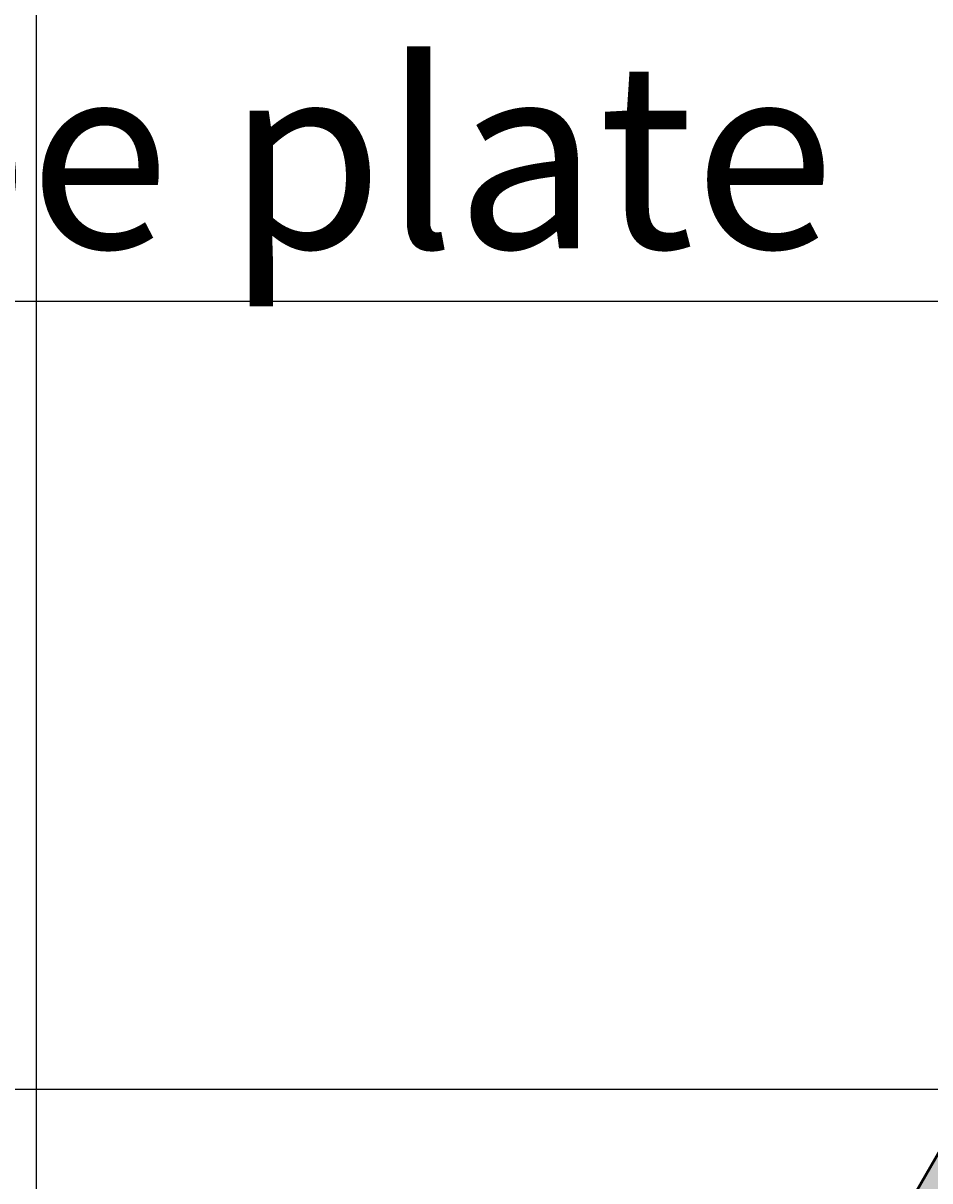
# Model space of a CAD drawing. Units: inches. Extents: x -12 to 334, y -10 to 186.
# Tile 59 of 77: x 106 to 125, y 136 to 161. Entities that reach past the tile are written whole.
import ezdxf
from ezdxf import colors
from ezdxf.entities.mleader import LeaderData, LeaderLine
from ezdxf.math import Vec2, Vec3

# ---------------------------------------------------------------- set-up
doc = ezdxf.new("R2010")
doc.units = ezdxf.units.IN
doc.header["$MEASUREMENT"] = 0
for name, color, linetype, lineweight in [('M-ANNO-TEXT', 3, 'Continuous', 25), ('M-DIMS', 2, 'Continuous', 18), ('M-EQPM', 7, 'Continuous', 50), ('M-EQPM-PATT', 8, 'Continuous', 18)]:
    doc.layers.add(name, color=color, linetype=linetype, lineweight=lineweight)
doc.styles.get("Standard").update_dxf_attribs({"font": 'arial.ttf'})
doc.dimstyles.get("Standard").update_dxf_attribs({"dimtxt": 0.18, "dimasz": 0.18, "dimexe": 0.18, "dimexo": 0.0625, "dimgap": 0.09, "dimtad": 0, "dimtih": 1, "dimtoh": 1, "dimdec": 4, "dimzin": 0, "dimdsep": 46, "dimtxsty": 'Standard', "dimcen": 0.09, "dimadec": 0, "dimazin": 0, "dimtfac": 1, "dimtdec": 4, "dimtofl": 0, "dimtmove": 0, "dimatfit": 3, "dimfxl": 1, "dimtolj": 1, "dimtzin": 0, "dimarcsym": 0})

# ---------------------------------------------------------------- blocks, each defined once
blk = doc.blocks.new('*D15')
at = {"layer": 'Defpoints', "color": 0, "transparency": 16777216}
for p in [(106.177, 169.385), (86.888, 109.058), (106.177, 102.896)]:
    blk.add_point(p, dxfattribs=at)
at = {"layer": 'M-DIMS', "color": 0, "lineweight": -2, "transparency": 16777216}
for p, q in [((86.888, 109.121), (86.888, 169.565)), ((87.068, 169.385), (96.147, 169.385)), ((105.997, 169.385), (96.918, 169.385)), ((106.177, 102.958), (106.177, 169.565))]:
    blk.add_line(p, q, dxfattribs=at)
at = {"layer": 'M-DIMS', "color": 0, "transparency": 16777216}
for points in [[(87.068, 169.415), (87.068, 169.355), (86.888, 169.385)], [(105.997, 169.415), (105.997, 169.355), (106.177, 169.385)]]:
    blk.add_solid(points, dxfattribs=at)
at = {"layer": 'M-DIMS', "color": 0, "transparency": 16777216, "insert": (96.532, 169.385), "char_height": 0.18, "attachment_point": 5}
blk.add_mtext('\\A1;19.29', dxfattribs=at)
blk = doc.blocks.new('*D16')
at = {"layer": 'Defpoints', "color": 0, "transparency": 16777216}
for p in [(126.379, 169.385), (126.379, 137.887), (106.177, 102.896)]:
    blk.add_point(p, dxfattribs=at)
at = {"layer": 'M-DIMS', "color": 0, "lineweight": -2, "transparency": 16777216}
for p, q in [((106.177, 102.958), (106.177, 169.565)), ((106.357, 169.385), (115.814, 169.385)), ((126.199, 169.385), (116.742, 169.385)), ((126.379, 137.95), (126.379, 169.565))]:
    blk.add_line(p, q, dxfattribs=at)
at = {"layer": 'M-DIMS', "color": 0, "transparency": 16777216}
for points in [[(106.357, 169.415), (106.357, 169.355), (106.177, 169.385)], [(126.199, 169.415), (126.199, 169.355), (126.379, 169.385)]]:
    blk.add_solid(points, dxfattribs=at)
at = {"layer": 'M-DIMS', "color": 0, "transparency": 16777216, "insert": (116.278, 169.385), "char_height": 0.18, "attachment_point": 5}
blk.add_mtext('\\A1;20.202', dxfattribs=at)
blk = doc.blocks.new('*D22')
at = {"layer": 'Defpoints', "color": 0, "transparency": 16777216}
for p in [(190.342, 154.835), (-11.174, 137.887), (195.342, 137.887)]:
    blk.add_point(p, dxfattribs=at)
at = {"layer": 'M-DIMS', "color": 0, "lineweight": -2, "transparency": 16777216}
for p, q in [((190.28, 154.835), (-11.354, 154.835)), ((-11.174, 154.655), (-11.174, 146.543)), ((-11.174, 138.067), (-11.174, 146.179)), ((195.28, 137.887), (-11.354, 137.887))]:
    blk.add_line(p, q, dxfattribs=at)
at = {"layer": 'M-DIMS', "color": 0, "transparency": 16777216}
for points in [[(-11.204, 154.655), (-11.144, 154.655), (-11.174, 154.835)], [(-11.204, 138.067), (-11.144, 138.067), (-11.174, 137.887)]]:
    blk.add_solid(points, dxfattribs=at)
at = {"layer": 'M-DIMS', "color": 0, "transparency": 16777216, "insert": (-11.174, 146.361), "char_height": 0.18, "attachment_point": 5}
blk.add_mtext('\\A1;16.947', dxfattribs=at)

msp = doc.modelspace()

# ---------------------------------------------------------------- hatches: boundary and pattern name
at = {"layer": 'M-EQPM-PATT'}
h = msp.add_hatch(color=256, dxfattribs=at)
h.set_gradient(color1=(99, 100, 102), color2=(99, 100, 102), tint=1)
h.paths.add_polyline_path([(126.9567, 136.8871), (179.7818, 136.8871), (180.0106, 137.8871), (126.3793, 137.8871), (106.1771, 102.8958), (86.8879, 102.8958), (86.8879, 109.0583), (84.7229, 109.0583), (84.7229, 100.8958), (106.1771, 100.8958)])
h.paths.add_polyline_path([(196.3421, 152.8345), (195.3421, 152.8345), (195.3421, 137.8871), (180.0106, 137.8871), (179.7818, 136.8871), (196.3421, 136.8871)])
h.paths.add_polyline_path([(215.0166, 152.8345), (214.0166, 152.8345), (214.0166, 136.9435), (268.3808, 136.9435, -0.2673785), (268.3808, 46.8541), (249.3759, 46.8541), (249.8485, 45.8541), (269.3808, 45.8541, 0.2615891), (269.3808, 137.9435), (215.0166, 137.9435)])

# ---------------------------------------------------------------- linework, layer by layer
at = {"layer": 'M-EQPM'}
msp.add_lwpolyline([(106.1771, 102.8958), (126.3793, 137.8871), (195.3421, 137.8871), (195.3421, 152.8345)], dxfattribs=at)

# ---------------------------------------------------------------- dimensions: what is measured, and where the dimension line sits
at = {"layer": 'M-DIMS'}
for base, p1, p2, override, picture, middle in [((106.1771, 169.3845), (86.8879, 109.0583), (106.1771, 102.8958), {"dimdec": 2, "dimlfac": 1, "dimrnd": 0, "dimzin": 0, "dimdsep": 46, "dimlunit": 2}, '*D15', (96.5325, 169.3845)), ((126.3793, 169.3845), (106.1771, 102.8958), (126.3793, 137.8871), {"dimdec": 3, "dimlfac": 1, "dimrnd": 0, "dimzin": 0, "dimdsep": 46, "dimlunit": 2}, '*D16', (116.2782, 169.3845))]:
    dim = msp.add_linear_dim(base=base, p1=p1, p2=p2, dimstyle='Standard', override=override, dxfattribs=at)
    dim.commit()
    dim.dimension.update_dxf_attribs({"geometry": picture, "text_midpoint": middle})
dim = msp.add_linear_dim(base=(-11.1736, 137.8871), p1=(190.3421, 154.8345), p2=(195.3421, 137.8871), angle=90, dimstyle='Standard', override={"dimdec": 3, "dimlfac": 1, "dimrnd": 0, "dimzin": 0, "dimdsep": 46, "dimlunit": 2}, dxfattribs=at)
dim.commit()
dim.dimension.update_dxf_attribs({"geometry": '*D22', "text_midpoint": (-11.1735, 146.3608)})

# ---------------------------------------------------------------- leaders
at = {"layer": 'M-ANNO-TEXT'}
ml = msp.add_multileader_mtext('Standard', dxfattribs=at)
ml.set_content('Tube plate', color=256)
ml.set_leader_properties()
ml.build(insert=Vec2(0, 0))
ml.multileader.update_dxf_attribs({"dogleg_length": 0.36, "arrow_head_size": 0.7})
ctx = ml.context
ctx.base_point, ctx.arrow_head_size, ctx.landing_gap_size, ctx.plane_origin = Vec3(95.9742, 157.4218), 0.7, 0.09, Vec3(31.4743, 171.7024)
notes = []
notes.append((ctx, [(0, (1, 1, 0), (78.5354, 157.4218), (1, 0), 17.4388, [(0, [(75.9244, 109.0583)], 0, [])])]))
ctx.mtext.insert, ctx.mtext.flow_direction = Vec3(96.0642, 159.9771), 5
for ctx, leaders in notes:
    for number, flags, end, landing, length, lines in leaders:
        leader = LeaderData()
        leader.index, (leader.has_last_leader_line, leader.has_dogleg_vector, leader.attachment_direction) = number, flags
        leader.last_leader_point, leader.dogleg_vector, leader.dogleg_length = Vec3(end), Vec3(landing), length
        for number, points, colour, breaks in lines:
            line = LeaderLine()
            line.index, line.vertices, line.color, line.breaks = number, Vec3.list(points), colors.encode_raw_color(colour), breaks
            leader.lines.append(line)
        ctx.leaders.append(leader)

doc.saveas('drawing.dxf')
